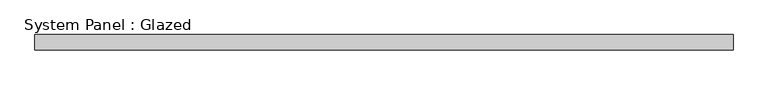
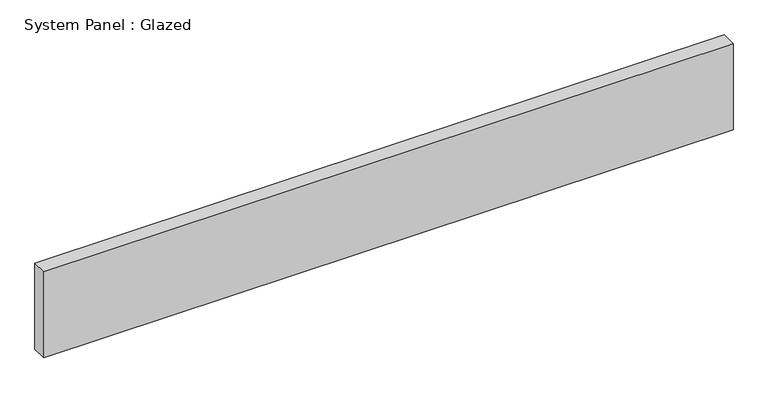
"""IFC4 building model written with IfcOpenShell, lengths in millimetres: plate geometry, System Panel : Glazed."""

from ifc_helpers import new_model, si_unit, origin, origin_with_axes, place, context, project, spatial, polyline, outline, extrude, source, transform, mapped, element, save


def system_panel_glazed_6c2d91e7(model_context):
    return source(origin(), model_context, "Body", "SweptSolid", [
        extrude(outline(polyline([(568.8031523, 24.5), (-568.8031523, 24.5), (-568.8031523, 49.5), (568.8031523, 49.5), (568.8031523, 24.5)])), origin_with_axes(), (0.0, 0.0, 1.0), 150.0429688),
    ])


if __name__ == "__main__":
    model = new_model("IFC4")
    model_context = context("Model", 3, world=origin())
    ifc_project = project(units=[si_unit("LENGTHUNIT", "METRE", prefix="MILLI")], contexts=[model_context])
    site = spatial("IfcSite", under=ifc_project)
    building = spatial("IfcBuilding", under=site)
    placement = place(None, origin())
    system_panel_glazed_shape = system_panel_glazed_6c2d91e7(model_context)
    element("IfcPlate", 1, ObjectType="System Panel : Glazed", at=placement, inside=building, context=model_context, shape_type="MappedRepresentation", body=[
        mapped(system_panel_glazed_shape, transform((0.0, 0.0, 0.0), x_axis=(1.0, 0.0, 0.0), y_axis=(0.0, 1.0, 0.0), z_axis=(0.0, 0.0, 1.0))),
    ])
    save(model, "model.ifc")

# Revit data of these elements
# Type "System Panel : Glazed"
#   Keynote = "H11"
#   Construction Type Id = "GSP4R"
#   Analytic Construction = "1/8 in Pilkington single glazing"
#   Visual Light Transmittance = 0.9
#   Solar Heat Gain Coefficient = 0.86
#   Heat Transfer Coefficient (U) = 6.7069 W/(m²·K)
#   Define Thermal Properties by = 1
# Element 1 (IfcPlate, "System Panel : Glazed")
#   Materials on its faces: "Glass"
# Materials
#   "Glass": class "Glass", colour RGB 0 128 192, transparency 0.9, Description = "Soda Lime Glass", Cost = 0
